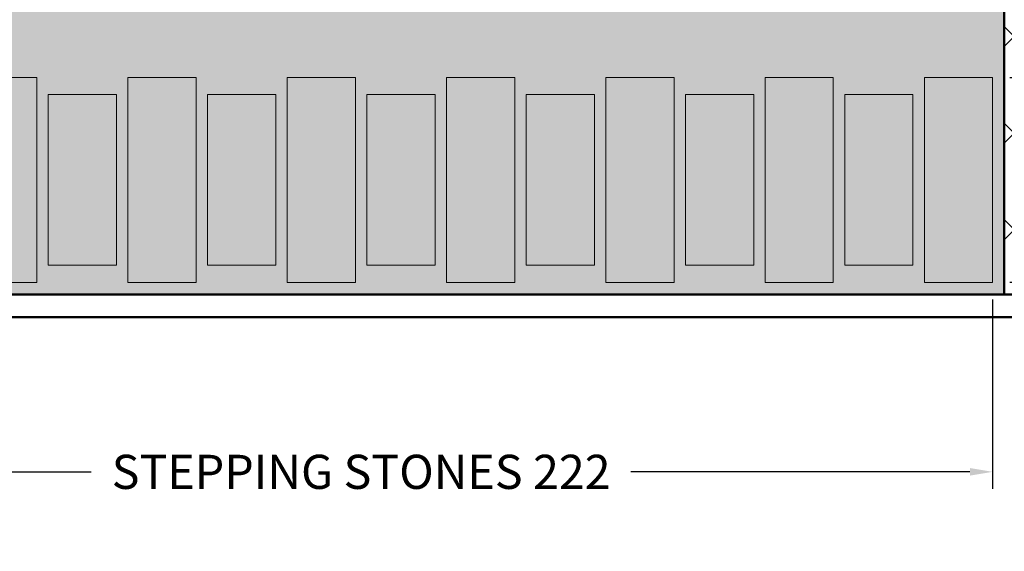
# Model space of a CAD drawing. Units: inches. Extents: x -466983 to 1020, y 324 to 318697.
# Tile 9 of 97: x 641 to 814, y 324 to 417. Entities that reach past the tile are written whole.
import ezdxf

# ---------------------------------------------------------------- set-up
doc = ezdxf.new("R2010")
doc.units = ezdxf.units.IN
doc.header["$MEASUREMENT"] = 0
for name, color, linetype, lineweight in [('A-ANNO-DIMS', 2, 'Continuous', 18), ('A-FLOR-PATT', 252, 'Continuous', 13), ('A-WALL', 7, 'Continuous', 50), ('L-SITE', 3, 'Continuous', 18)]:
    doc.layers.add(name, color=color, linetype=linetype, lineweight=lineweight)
doc.layers.add('K-Hatch', color=7, linetype='Continuous')
doc.styles.get("Standard").update_dxf_attribs({"font": 'arial.ttf'})
doc.dimstyles.get("Standard").update_dxf_attribs({"dimtxt": 6, "dimasz": 4, "dimexe": 3, "dimexo": 3, "dimgap": 0.09, "dimtad": 0, "dimtih": 1, "dimtoh": 1, "dimdec": 1, "dimzin": 0, "dimdsep": 46, "dimlunit": 3, "dimtxsty": 'Standard', "dimcen": 0.09, "dimadec": 0, "dimazin": 0, "dimtfac": 1, "dimtdec": 1, "dimtofl": 0, "dimtmove": 0, "dimatfit": 3, "dimfxl": 1, "dimtolj": 1, "dimtzin": 0, "dimarcsym": 0})

# ---------------------------------------------------------------- blocks, each defined once
blk = doc.blocks.new('Garden stone')
at = {"layer": 'K-Hatch'}
h = blk.add_hatch(color=256, dxfattribs=at)
h.dxf.hatch_style = 1
h.set_gradient(color1=(254, 234, 185), color2=(128, 128, 128), name='CYLINDER')
h.paths.add_polyline_path([(1856.21, 697.1), (1844.21, 697.1), (1844.21, 661.1), (1856.21, 661.1)])
h = blk.add_hatch(color=256, dxfattribs=at)
h.dxf.hatch_style = 1
h.set_gradient(color1=(254, 234, 185), color2=(128, 128, 128), name='CYLINDER')
h.paths.add_polyline_path([(1884.21, 697.1), (1872.21, 697.1), (1872.21, 661.1), (1884.21, 661.1)])
h = blk.add_hatch(color=256, dxfattribs=at)
h.dxf.hatch_style = 1
h.set_gradient(color1=(254, 234, 185), color2=(128, 128, 128), name='CYLINDER')
h.paths.add_polyline_path([(1912.21, 697.1), (1900.21, 697.1), (1900.21, 661.1), (1912.21, 661.1)])
h = blk.add_hatch(color=256, dxfattribs=at)
h.dxf.hatch_style = 1
h.set_gradient(color1=(254, 234, 185), color2=(128, 128, 128), name='CYLINDER')
h.paths.add_polyline_path([(1940.21, 697.1), (1928.21, 697.1), (1928.21, 661.1), (1940.21, 661.1)])
h = blk.add_hatch(color=256, dxfattribs=at)
h.dxf.hatch_style = 1
h.set_gradient(color1=(254, 234, 185), color2=(128, 128, 128), name='CYLINDER')
h.paths.add_polyline_path([(1968.21, 697.1), (1956.21, 697.1), (1956.21, 661.1), (1968.21, 661.1)])
h = blk.add_hatch(color=256, dxfattribs=at)
h.dxf.hatch_style = 1
h.set_gradient(color1=(254, 234, 185), color2=(128, 128, 128), name='CYLINDER')
h.paths.add_polyline_path([(1996.21, 697.1), (1984.21, 697.1), (1984.21, 661.1), (1996.21, 661.1)])
h = blk.add_hatch(color=256, dxfattribs=at)
h.dxf.hatch_style = 1
h.set_gradient(color1=(254, 234, 185), color2=(128, 128, 128), name='CYLINDER')
h.paths.add_polyline_path([(2024.21, 697.1), (2012.21, 697.1), (2012.21, 661.1), (2024.21, 661.1)])
h = blk.add_hatch(color=256, dxfattribs=at)
h.dxf.hatch_style = 1
h.set_gradient(color1=(254, 234, 185), color2=(128, 128, 128), name='SPHERICAL')
h.paths.add_polyline_path([(1870.21, 694.1), (1858.21, 694.1), (1858.21, 664.1), (1870.21, 664.1)])
h = blk.add_hatch(color=256, dxfattribs=at)
h.dxf.hatch_style = 1
h.set_gradient(color1=(254, 234, 185), color2=(128, 128, 128), name='SPHERICAL')
h.paths.add_polyline_path([(1898.21, 694.1), (1886.21, 694.1), (1886.21, 664.1), (1898.21, 664.1)])
h = blk.add_hatch(color=256, dxfattribs=at)
h.dxf.hatch_style = 1
h.set_gradient(color1=(254, 234, 185), color2=(128, 128, 128), name='SPHERICAL')
h.paths.add_polyline_path([(1926.21, 694.1), (1914.21, 694.1), (1914.21, 664.1), (1926.21, 664.1)])
h = blk.add_hatch(color=256, dxfattribs=at)
h.dxf.hatch_style = 1
h.set_gradient(color1=(254, 234, 185), color2=(128, 128, 128), name='SPHERICAL')
h.paths.add_polyline_path([(1954.21, 694.1), (1942.21, 694.1), (1942.21, 664.1), (1954.21, 664.1)])
h = blk.add_hatch(color=256, dxfattribs=at)
h.dxf.hatch_style = 1
h.set_gradient(color1=(254, 234, 185), color2=(128, 128, 128), name='SPHERICAL')
h.paths.add_polyline_path([(1982.21, 694.1), (1970.21, 694.1), (1970.21, 664.1), (1982.21, 664.1)])
h = blk.add_hatch(color=256, dxfattribs=at)
h.dxf.hatch_style = 1
h.set_gradient(color1=(254, 234, 185), color2=(128, 128, 128), name='SPHERICAL')
h.paths.add_polyline_path([(2010.21, 694.1), (1998.21, 694.1), (1998.21, 664.1), (2010.21, 664.1)])
for points in [[(1844.21, 697.1), (1856.21, 697.1), (1856.21, 661.1), (1844.21, 661.1)], [(1872.21, 697.1), (1884.21, 697.1), (1884.21, 661.1), (1872.21, 661.1)], [(1900.21, 697.1), (1912.21, 697.1), (1912.21, 661.1), (1900.21, 661.1)], [(1928.21, 697.1), (1940.21, 697.1), (1940.21, 661.1), (1928.21, 661.1)], [(1956.21, 697.1), (1968.21, 697.1), (1968.21, 661.1), (1956.21, 661.1)], [(1984.21, 697.1), (1996.21, 697.1), (1996.21, 661.1), (1984.21, 661.1)], [(2012.21, 697.1), (2024.21, 697.1), (2024.21, 661.1), (2012.21, 661.1)], [(1858.21, 694.1), (1870.21, 694.1), (1870.21, 664.1), (1858.21, 664.1)], [(1886.21, 694.1), (1898.21, 694.1), (1898.21, 664.1), (1886.21, 664.1)], [(1914.21, 694.1), (1926.21, 694.1), (1926.21, 664.1), (1914.21, 664.1)], [(1942.21, 694.1), (1954.21, 694.1), (1954.21, 664.1), (1942.21, 664.1)], [(1970.21, 694.1), (1982.21, 694.1), (1982.21, 664.1), (1970.21, 664.1)], [(1998.21, 694.1), (2010.21, 694.1), (2010.21, 664.1), (1998.21, 664.1)]]:
    blk.add_lwpolyline(points, close=True)
blk = doc.blocks.new('*D115')
at = {"layer": 'A-ANNO-DIMS', "color": 0, "lineweight": -2, "transparency": 16777216}
for p, q in [((589.8, 368.07), (589.8, 334.77)), ((811.8, 368.07), (811.8, 334.77)), ((593.8, 337.77), (653.37, 337.77)), ((807.8, 337.77), (748.22, 337.77))]:
    blk.add_line(p, q, dxfattribs=at)
at = {"layer": 'A-ANNO-DIMS', "color": 0, "transparency": 16777216}
for points in [[(593.8, 338.44), (593.8, 337.1), (589.8, 337.77)], [(807.8, 338.44), (807.8, 337.1), (811.8, 337.77)]]:
    blk.add_solid(points, dxfattribs=at)
at = {"layer": 'Defpoints', "color": 0, "transparency": 16777216}
for p in [(589.8, 371.07), (811.8, 371.07), (811.8, 337.77)]:
    blk.add_point(p, dxfattribs=at)
at = {"layer": 'A-ANNO-DIMS', "color": 0, "transparency": 16777216, "insert": (700.8, 337.77), "char_height": 6, "attachment_point": 5}
blk.add_mtext('\\A1;STEPPING STONES 222', dxfattribs=at)
blk = doc.blocks.new('*D116')
at = {"layer": 'A-ANNO-DIMS', "color": 0, "lineweight": -2, "transparency": 16777216}
for p, q in [((814.8, 407.07), (848.1, 407.07)), ((845.1, 403.07), (845.1, 392.23)), ((845.1, 375.07), (845.1, 385.91)), ((814.8, 371.07), (848.1, 371.07))]:
    blk.add_line(p, q, dxfattribs=at)
at = {"layer": 'A-ANNO-DIMS', "color": 0, "transparency": 16777216}
for points in [[(844.43, 403.07), (845.76, 403.07), (845.1, 407.07)], [(844.43, 375.07), (845.76, 375.07), (845.1, 371.07)]]:
    blk.add_solid(points, dxfattribs=at)
at = {"layer": 'Defpoints', "color": 0, "transparency": 16777216}
for p in [(811.8, 407.07), (845.1, 407.07), (811.8, 371.07)]:
    blk.add_point(p, dxfattribs=at)
at = {"layer": 'A-ANNO-DIMS', "color": 0, "transparency": 16777216, "insert": (845.1, 389.07), "char_height": 6, "attachment_point": 5}
blk.add_mtext('\\A1;36', dxfattribs=at)

msp = doc.modelspace()

# ---------------------------------------------------------------- hatches: boundary and pattern name
at = {"layer": 'A-FLOR-PATT', "transparency": 33554572}
h = msp.add_hatch(dxfattribs=at)
h.set_pattern_fill('AR-HBONE', color=256, scale=3)
h.set_pattern_definition([(45, (-1212.414, -290.035), (0, 16.97056), [36, -12]), (135, (-1203.928, -281.55), (1e-15, 16.97056), [36, -12])])
h.paths.add_polyline_path([(987.81, 618.94), (813.81, 618.94), (813.81, 368.94), (987.81, 368.94)])
at = {"layer": 'A-FLOR-PATT', "transparency": 33554661}
h = msp.add_hatch(color=256, dxfattribs=at)
h.dxf.hatch_style = 1
h.set_gradient(color1=(19, 155, 72), color2=(0, 107, 0), name='CYLINDER')
h.paths.add_polyline_path([(813.81, 503.94), (730.81, 503.94), (730.81, 424.94), (612.81, 424.94), (612.81, 415.94), (442.81, 415.94), (442.81, 368.94), (813.81, 368.94)])
h.paths.add_polyline_path([(771.8, 407.07), (783.8, 407.07), (783.8, 371.07), (771.8, 371.07)], flags=16)
h.paths.add_polyline_path([(755.8, 407.07), (755.8, 371.07), (743.8, 371.07), (743.8, 407.07)], flags=16)
h.paths.add_polyline_path([(769.8, 404.07), (769.8, 374.07), (757.8, 374.07), (757.8, 404.07)], flags=16)
h.paths.add_polyline_path([(785.8, 404.07), (797.8, 404.07), (797.8, 374.07), (785.8, 374.07)], flags=16)
h.paths.add_polyline_path([(741.8, 404.07), (741.8, 374.07), (729.8, 374.07), (729.8, 404.07)], flags=16)
h.paths.add_polyline_path([(799.8, 407.07), (811.8, 407.07), (811.8, 371.07), (799.8, 371.07)], flags=16)
h.paths.add_polyline_path([(727.8, 407.07), (727.8, 371.07), (715.8, 371.07), (715.8, 407.07)], flags=16)
h.paths.add_polyline_path([(713.8, 404.07), (713.8, 374.07), (701.8, 374.07), (701.8, 404.07)], flags=16)
h.paths.add_polyline_path([(699.8, 407.07), (699.8, 371.07), (687.8, 371.07), (687.8, 407.07)], flags=16)
h.paths.add_polyline_path([(685.8, 404.07), (685.8, 374.07), (673.8, 374.07), (673.8, 404.07)], flags=16)
h.paths.add_polyline_path([(671.8, 407.07), (671.8, 371.07), (659.8, 371.07), (659.8, 407.07)], flags=16)
h.paths.add_polyline_path([(657.8, 404.07), (657.8, 374.07), (645.8, 374.07), (645.8, 404.07)], flags=16)
h.paths.add_polyline_path([(643.8, 407.07), (643.8, 371.07), (631.8, 371.07), (631.8, 407.07)], flags=16)
h.paths.add_polyline_path([(629.8, 404.07), (629.8, 374.07), (617.8, 374.07), (617.8, 404.07)], flags=16)
h.paths.add_polyline_path([(615.8, 407.07), (615.8, 371.07), (603.8, 371.07), (603.8, 407.07)], flags=16)
h.paths.add_polyline_path([(601.8, 404.07), (601.8, 374.07), (589.8, 374.07), (589.8, 404.07)], flags=16)
at = {"layer": 'A-FLOR-PATT'}
h = msp.add_hatch(dxfattribs=at)
h.set_pattern_fill('GRASS', color=256, scale=6)
h.set_pattern_definition([(90, (-1212.4137, -290.035), (-4.242641, 4.242641), [1.125, -7.360281]), (45, (-1212.4137, -290.035), (-4.24264, 4.24264), [1.125, -4.875]), (135, (-1212.4137, -290.035), (-4.24264, -4.24264), [1.125, -4.875])])
h.paths.add_polyline_path([(813.81, 503.94), (730.81, 503.94), (730.81, 424.94), (612.81, 424.94), (612.81, 415.94), (442.81, 415.94), (442.81, 368.94), (813.81, 368.94)])
h.paths.add_polyline_path([(589.8, 404.07), (601.8, 404.07), (601.8, 374.07), (589.8, 374.07)], flags=16)
h.paths.add_polyline_path([(603.8, 407.07), (615.8, 407.07), (615.8, 371.07), (603.8, 371.07)], flags=16)
h.paths.add_polyline_path([(617.8, 404.07), (629.8, 404.07), (629.8, 374.07), (617.8, 374.07)], flags=16)
h.paths.add_polyline_path([(631.8, 407.07), (643.8, 407.07), (643.8, 371.07), (631.8, 371.07)], flags=16)
h.paths.add_polyline_path([(645.8, 404.07), (657.8, 404.07), (657.8, 374.07), (645.8, 374.07)], flags=16)
h.paths.add_polyline_path([(659.8, 407.07), (671.8, 407.07), (671.8, 371.07), (659.8, 371.07)], flags=16)
h.paths.add_polyline_path([(673.8, 404.07), (685.8, 404.07), (685.8, 374.07), (673.8, 374.07)], flags=16)
h.paths.add_polyline_path([(687.8, 407.07), (699.8, 407.07), (699.8, 371.07), (687.8, 371.07)], flags=16)
h.paths.add_polyline_path([(701.8, 404.07), (713.8, 404.07), (713.8, 374.07), (701.8, 374.07)], flags=16)
h.paths.add_polyline_path([(715.8, 407.07), (727.8, 407.07), (727.8, 371.07), (715.8, 371.07)], flags=16)
h.paths.add_polyline_path([(729.8, 404.07), (741.8, 404.07), (741.8, 374.07), (729.8, 374.07)], flags=16)
h.paths.add_polyline_path([(743.8, 407.07), (755.8, 407.07), (755.8, 371.07), (743.8, 371.07)], flags=16)
h.paths.add_polyline_path([(757.8, 404.07), (769.8, 404.07), (769.8, 374.07), (757.8, 374.07)], flags=16)
h.paths.add_polyline_path([(771.8, 407.07), (783.8, 407.07), (783.8, 371.07), (771.8, 371.07)], flags=16)
h.paths.add_polyline_path([(785.8, 404.07), (797.8, 404.07), (797.8, 374.07), (785.8, 374.07)], flags=16)
h.paths.add_polyline_path([(799.8, 407.07), (811.8, 407.07), (811.8, 371.07), (799.8, 371.07)], flags=16)

# ---------------------------------------------------------------- linework, layer by layer
at = {"layer": 'A-WALL'}
for p, q in [((813.81, 618.94), (813.81, 368.94)), ((987.81, 368.94), (395.81, 368.94)), ((991.81, 364.94), (391.81, 364.94))]:
    msp.add_line(p, q, dxfattribs=at)

# ---------------------------------------------------------------- block references
at = {"layer": 'L-SITE'}
msp.add_blockref('Garden stone', (-1212.41, -290.04), dxfattribs=at)

# ---------------------------------------------------------------- dimensions: what is measured, and where the dimension line sits
at = {"layer": 'A-ANNO-DIMS'}
dim = msp.add_linear_dim(base=(845.1, 407.07), p1=(811.8, 371.07), p2=(811.8, 407.07), angle=90, dimstyle='Standard', override={"dimdec": 0, "dimlfac": 1, "dimrnd": 0, "dimzin": 0, "dimdsep": 46, "dimlunit": 2}, dxfattribs=at)
dim.commit()
dim.dimension.update_dxf_attribs({"geometry": '*D116', "text_midpoint": (845.1, 389.07)})
dim = msp.add_linear_dim(base=(811.8, 337.77), p1=(589.8, 371.07), p2=(811.8, 371.07), text='STEPPING STONES <>', dimstyle='Standard', override={"dimdec": 0, "dimlfac": 1, "dimrnd": 0, "dimzin": 0, "dimdsep": 46, "dimlunit": 2}, dxfattribs=at)
dim.commit()
dim.dimension.update_dxf_attribs({"geometry": '*D115', "text_midpoint": (700.8, 337.77)})

doc.saveas('drawing.dxf')
